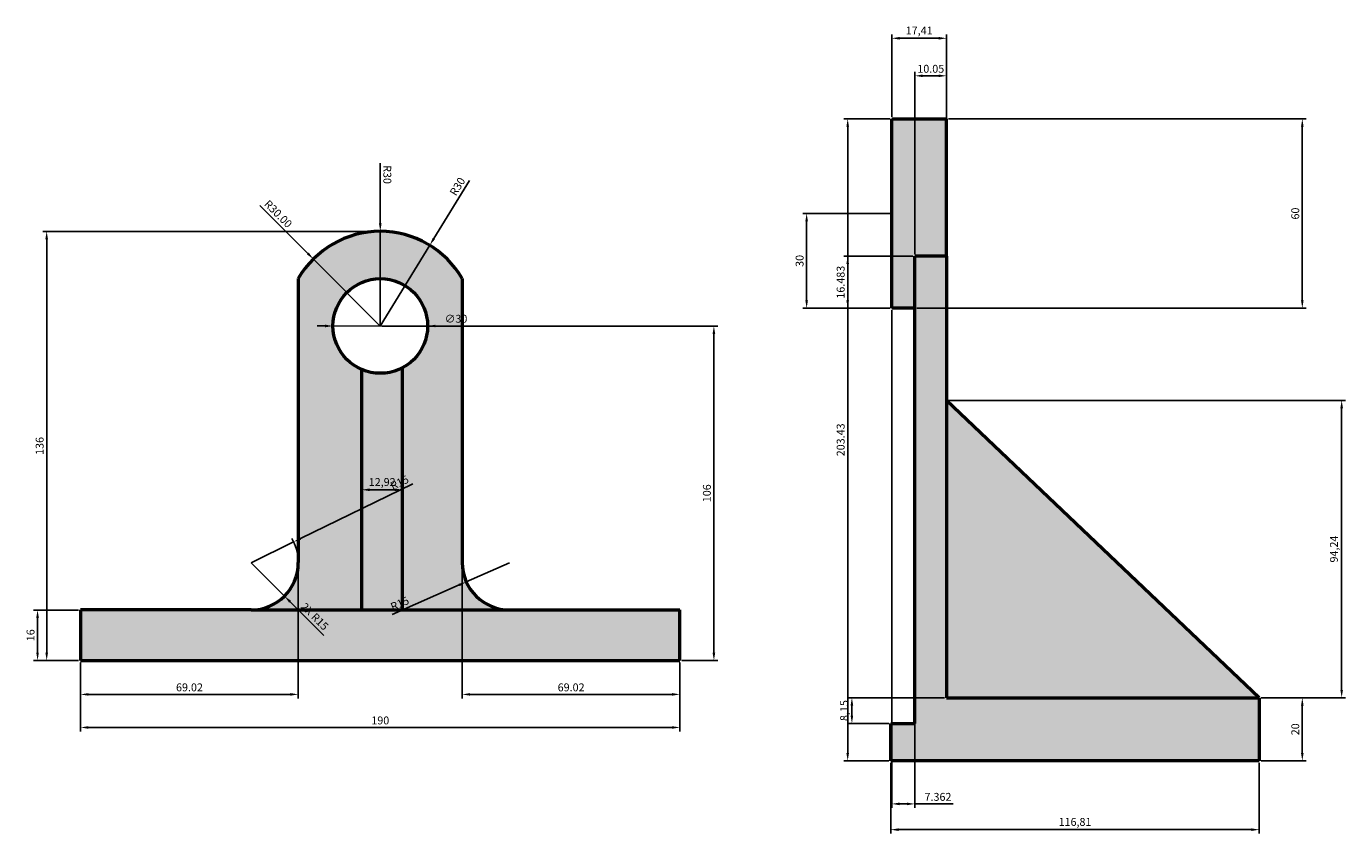
# Model space of a CAD drawing. Units: millimetres. Extents: x 1248 to 2192, y 1962 to 2325.
# Tile 4 of 4: x 1773 to 2192, y 2069 to 2325. Entities that reach past the tile are written whole.
import ezdxf

# ---------------------------------------------------------------- set-up
doc = ezdxf.new("R2010")
doc.units = ezdxf.units.MM
for name, color, linetype, lineweight in [('M-DIMS', 2, 'Continuous', 25), ('M-HATC', 8, 'Continuous', 18), ('M-OUTL', 7, 'Continuous', 50)]:
    doc.layers.add(name, color=color, linetype=linetype, lineweight=lineweight)
doc.styles.get("Standard").update_dxf_attribs({"font": 'arial.ttf'})
doc.dimstyles.new('ISO-25', dxfattribs={"dimtxt": 2.5, "dimasz": 2.5, "dimexe": 1.25, "dimexo": 0.625, "dimtad": 1, "dimtxsty": 'Standard', "dimcen": 2.5, "dimadec": 0, "dimazin": 0, "dimtfac": 1, "dimtmove": 0, "dimatfit": 3, "dimfxl": 1, "dimarcsym": 0})

# ---------------------------------------------------------------- blocks, each defined once
blk = doc.blocks.new('*D23')
at = {"layer": 'Defpoints', "color": 0, "transparency": 16777216}
for p in [(1790.51, 2124.07), (1980.51, 2124.07), (1980.51, 2102.85)]:
    blk.add_point(p, dxfattribs=at)
at = {"layer": 'M-DIMS', "color": 0, "lineweight": -2, "transparency": 16777216}
for p, q in [((1790.51, 2123.45), (1790.51, 2101.6)), ((1980.51, 2123.45), (1980.51, 2101.6)), ((1793.01, 2102.85), (1978.01, 2102.85))]:
    blk.add_line(p, q, dxfattribs=at)
at = {"layer": 'M-DIMS', "color": 0, "transparency": 16777216}
for points in [[(1793.01, 2103.26), (1793.01, 2102.43), (1790.51, 2102.85)], [(1978.01, 2103.26), (1978.01, 2102.43), (1980.51, 2102.85)]]:
    blk.add_solid(points, dxfattribs=at)
at = {"layer": 'M-DIMS', "color": 0, "transparency": 16777216, "insert": (1885.51, 2104.75), "char_height": 2.5, "attachment_point": 5}
blk.add_mtext('190', dxfattribs=at)
blk = doc.blocks.new('*D24')
at = {"layer": 'Defpoints', "color": 0, "transparency": 16777216}
for p in [(1776.87, 2140.07), (1790.51, 2140.07), (1790.51, 2124.07)]:
    blk.add_point(p, dxfattribs=at)
at = {"layer": 'M-DIMS', "color": 0, "lineweight": -2, "transparency": 16777216}
for p, q in [((1789.89, 2140.07), (1775.62, 2140.07)), ((1776.87, 2126.57), (1776.87, 2137.57)), ((1789.89, 2124.07), (1775.62, 2124.07))]:
    blk.add_line(p, q, dxfattribs=at)
at = {"layer": 'M-DIMS', "color": 0, "transparency": 16777216}
for points in [[(1776.45, 2137.57), (1777.28, 2137.57), (1776.87, 2140.07)], [(1776.45, 2126.57), (1777.28, 2126.57), (1776.87, 2124.07)]]:
    blk.add_solid(points, dxfattribs=at)
at = {"layer": 'M-DIMS', "color": 0, "transparency": 16777216, "insert": (1774.97, 2132.07), "char_height": 2.5, "attachment_point": 5, "rotation": 90}
blk.add_mtext('16', dxfattribs=at)
blk = doc.blocks.new('*D25')
at = {"layer": 'Defpoints', "color": 0, "transparency": 16777216}
for p in [(1901.18, 2255.66), (1885.51, 2230.07)]:
    blk.add_point(p, dxfattribs=at)
at = {"layer": 'M-DIMS', "color": 0, "lineweight": -2, "transparency": 16777216}
for p, q in [((1913.76, 2276.19), (1902.49, 2257.79)), ((1885.51, 2230.07), (1901.18, 2255.66))]:
    blk.add_line(p, q, dxfattribs=at)
at = {"layer": 'M-DIMS', "color": 0, "transparency": 16777216}
blk.add_solid([(1902.13, 2258.01), (1902.84, 2257.57), (1901.18, 2255.66)], dxfattribs=at)
at = {"layer": 'M-DIMS', "color": 0, "transparency": 16777216, "insert": (1910.25, 2274.11), "char_height": 2.5, "attachment_point": 5, "rotation": 58.5121}
blk.add_mtext('R30', dxfattribs=at)
blk = doc.blocks.new('*D26')
at = {"layer": 'Defpoints', "color": 0, "transparency": 16777216}
for p in [(1858.02, 2161.64), (1844.53, 2155.07)]:
    blk.add_point(p, dxfattribs=at)
at = {"layer": 'M-DIMS', "color": 0, "lineweight": -2, "transparency": 16777216}
for p, q in [((1895.83, 2180.04), (1860.26, 2162.73)), ((1844.53, 2155.07), (1858.02, 2161.64))]:
    blk.add_line(p, q, dxfattribs=at)
blk.add_arc((1844.53, 2155.07), 15, 2.3873, 30.7269, dxfattribs=at)
at = {"layer": 'M-DIMS', "color": 0, "transparency": 16777216}
blk.add_solid([(1860.08, 2163.11), (1860.45, 2162.36), (1858.02, 2161.64)], dxfattribs=at)
at = {"layer": 'M-DIMS', "color": 0, "transparency": 16777216, "insert": (1891.74, 2180.17), "char_height": 2.5, "attachment_point": 5, "rotation": 25.9523}
blk.add_mtext('R15', dxfattribs=at)
blk = doc.blocks.new('*D27')
at = {"layer": 'Defpoints', "color": 0, "transparency": 16777216}
for p in [(1926.49, 2155.07), (1912.77, 2149.01)]:
    blk.add_point(p, dxfattribs=at)
at = {"layer": 'M-DIMS', "color": 0, "lineweight": -2, "transparency": 16777216}
for p, q in [((1926.49, 2155.07), (1912.77, 2149.01)), ((1889.26, 2138.61), (1910.49, 2148))]:
    blk.add_line(p, q, dxfattribs=at)
at = {"layer": 'M-DIMS', "color": 0, "transparency": 16777216}
blk.add_solid([(1910.32, 2148.38), (1910.65, 2147.61), (1912.77, 2149.01)], dxfattribs=at)
at = {"layer": 'M-DIMS', "color": 0, "transparency": 16777216, "insert": (1891.81, 2141.81), "char_height": 2.5, "attachment_point": 5, "rotation": 23.8585}
blk.add_mtext('R15', dxfattribs=at)
blk = doc.blocks.new('*D28')
at = {"layer": 'Defpoints', "color": 0, "transparency": 16777216}
for p in [(1879.65, 2178.17), (1892.58, 2178.46), (1892.58, 2178.17)]:
    blk.add_point(p, dxfattribs=at)
at = {"layer": 'M-DIMS', "color": 0, "lineweight": -2, "transparency": 16777216}
for p, q in [((1879.65, 2178.8), (1879.65, 2179.42)), ((1882.15, 2178.17), (1890.08, 2178.17)), ((1892.58, 2177.83), (1892.58, 2176.92))]:
    blk.add_line(p, q, dxfattribs=at)
at = {"layer": 'M-DIMS', "color": 0, "transparency": 16777216}
for points in [[(1882.15, 2178.59), (1882.15, 2177.75), (1879.65, 2178.17)], [(1890.08, 2178.59), (1890.08, 2177.75), (1892.58, 2178.17)]]:
    blk.add_solid(points, dxfattribs=at)
at = {"layer": 'M-DIMS', "color": 0, "transparency": 16777216, "insert": (1886.11, 2180.3), "char_height": 2.5, "attachment_point": 5}
blk.add_mtext('12,92', dxfattribs=at)
blk = doc.blocks.new('*D29')
at = {"layer": 'Defpoints', "color": 0, "transparency": 16777216}
for p in [(2065.03, 2321.25), (2047.62, 2295.71), (2065.03, 2295.71)]:
    blk.add_point(p, dxfattribs=at)
at = {"layer": 'M-DIMS', "color": 0, "lineweight": -2, "transparency": 16777216}
for p, q in [((2047.62, 2296.33), (2047.62, 2322.5)), ((2050.12, 2321.25), (2062.53, 2321.25)), ((2065.03, 2296.33), (2065.03, 2322.5))]:
    blk.add_line(p, q, dxfattribs=at)
at = {"layer": 'M-DIMS', "color": 0, "transparency": 16777216}
for points in [[(2050.12, 2321.67), (2050.12, 2320.83), (2047.62, 2321.25)], [(2062.53, 2321.67), (2062.53, 2320.83), (2065.03, 2321.25)]]:
    blk.add_solid(points, dxfattribs=at)
at = {"layer": 'M-DIMS', "color": 0, "transparency": 16777216, "insert": (2056.32, 2323.38), "char_height": 2.5, "attachment_point": 5}
blk.add_mtext('17,41', dxfattribs=at)
blk = doc.blocks.new('*D30')
at = {"layer": 'Defpoints', "color": 0, "transparency": 16777216}
for p in [(2047.62, 2265.71), (2020.66, 2235.71), (2047.62, 2235.71)]:
    blk.add_point(p, dxfattribs=at)
at = {"layer": 'M-DIMS', "color": 0, "lineweight": -2, "transparency": 16777216}
for p, q in [((2046.99, 2265.71), (2019.41, 2265.71)), ((2020.66, 2263.21), (2020.66, 2238.21)), ((2046.99, 2235.71), (2019.41, 2235.71))]:
    blk.add_line(p, q, dxfattribs=at)
at = {"layer": 'M-DIMS', "color": 0, "transparency": 16777216}
for points in [[(2020.25, 2263.21), (2021.08, 2263.21), (2020.66, 2265.71)], [(2020.25, 2238.21), (2021.08, 2238.21), (2020.66, 2235.71)]]:
    blk.add_solid(points, dxfattribs=at)
at = {"layer": 'M-DIMS', "color": 0, "transparency": 16777216, "insert": (2018.76, 2250.71), "char_height": 2.5, "attachment_point": 5, "rotation": 90}
blk.add_mtext('30', dxfattribs=at)
blk = doc.blocks.new('*D31')
at = {"layer": 'Defpoints', "color": 0, "transparency": 16777216}
for p in [(2065.03, 2206.51), (2164.13, 2112.27), (2190.26, 2112.27)]:
    blk.add_point(p, dxfattribs=at)
at = {"layer": 'M-DIMS', "color": 0, "lineweight": -2, "transparency": 16777216}
for p, q in [((2065.66, 2206.51), (2191.51, 2206.51)), ((2190.26, 2204.01), (2190.26, 2114.77)), ((2164.76, 2112.27), (2191.51, 2112.27))]:
    blk.add_line(p, q, dxfattribs=at)
at = {"layer": 'M-DIMS', "color": 0, "transparency": 16777216}
for points in [[(2189.85, 2204.01), (2190.68, 2204.01), (2190.26, 2206.51)], [(2189.85, 2114.77), (2190.68, 2114.77), (2190.26, 2112.27)]]:
    blk.add_solid(points, dxfattribs=at)
at = {"layer": 'M-DIMS', "color": 0, "transparency": 16777216, "insert": (2188.13, 2159.39), "char_height": 2.5, "attachment_point": 5, "rotation": 90}
blk.add_mtext('94,24', dxfattribs=at)
blk = doc.blocks.new('*D32')
at = {"layer": 'Defpoints', "color": 0, "transparency": 16777216}
for p in [(2047.32, 2092.27), (2164.13, 2092.27), (2164.13, 2070.46)]:
    blk.add_point(p, dxfattribs=at)
at = {"layer": 'M-DIMS', "color": 0, "lineweight": -2, "transparency": 16777216}
for p, q in [((2047.32, 2091.65), (2047.32, 2069.21)), ((2164.13, 2091.65), (2164.13, 2069.21)), ((2049.82, 2070.46), (2161.63, 2070.46))]:
    blk.add_line(p, q, dxfattribs=at)
at = {"layer": 'M-DIMS', "color": 0, "transparency": 16777216}
for points in [[(2049.82, 2070.88), (2049.82, 2070.04), (2047.32, 2070.46)], [(2161.63, 2070.88), (2161.63, 2070.04), (2164.13, 2070.46)]]:
    blk.add_solid(points, dxfattribs=at)
at = {"layer": 'M-DIMS', "color": 0, "transparency": 16777216, "insert": (2105.73, 2072.59), "char_height": 2.5, "attachment_point": 5}
blk.add_mtext('116,81', dxfattribs=at)
blk = doc.blocks.new('*D33')
at = {"layer": 'Defpoints', "color": 0, "transparency": 16777216}
for p in [(2035.01, 2112.27), (2065.03, 2112.27), (2047.32, 2104.13)]:
    blk.add_point(p, dxfattribs=at)
at = {"layer": 'M-DIMS', "color": 0, "lineweight": -2, "transparency": 16777216}
for p, q in [((2064.41, 2112.27), (2033.76, 2112.27)), ((2035.01, 2106.63), (2035.01, 2109.77)), ((2046.7, 2104.13), (2033.76, 2104.13))]:
    blk.add_line(p, q, dxfattribs=at)
at = {"layer": 'M-DIMS', "color": 0, "transparency": 16777216}
for points in [[(2034.59, 2109.77), (2035.42, 2109.77), (2035.01, 2112.27)], [(2034.59, 2106.63), (2035.42, 2106.63), (2035.01, 2104.13)]]:
    blk.add_solid(points, dxfattribs=at)
at = {"layer": 'M-DIMS', "color": 0, "transparency": 16777216, "insert": (2032.88, 2108.2), "char_height": 2.5, "attachment_point": 5, "rotation": 90}
blk.add_mtext('8,15', dxfattribs=at)
blk = doc.blocks.new('*D34')
at = {"layer": 'Defpoints', "color": 0, "transparency": 16777216}
for p in [(1779.76, 2260.07), (1885.51, 2260.07), (1790.51, 2124.07)]:
    blk.add_point(p, dxfattribs=at)
at = {"layer": 'M-DIMS', "color": 0, "lineweight": -2, "transparency": 16777216}
for p, q in [((1884.89, 2260.07), (1778.51, 2260.07)), ((1779.76, 2126.57), (1779.76, 2257.57)), ((1789.89, 2124.07), (1778.51, 2124.07))]:
    blk.add_line(p, q, dxfattribs=at)
at = {"layer": 'M-DIMS', "color": 0, "transparency": 16777216}
for points in [[(1779.34, 2257.57), (1780.18, 2257.57), (1779.76, 2260.07)], [(1779.34, 2126.57), (1780.18, 2126.57), (1779.76, 2124.07)]]:
    blk.add_solid(points, dxfattribs=at)
at = {"layer": 'M-DIMS', "color": 0, "transparency": 16777216, "insert": (1777.86, 2192.07), "char_height": 2.5, "attachment_point": 5, "rotation": 90}
blk.add_mtext('136', dxfattribs=at)
blk = doc.blocks.new('*D35')
at = {"layer": 'Defpoints', "color": 0, "transparency": 16777216}
for p in [(1885.51, 2230.07), (1991.26, 2230.07), (1980.51, 2124.07)]:
    blk.add_point(p, dxfattribs=at)
at = {"layer": 'M-DIMS', "color": 0, "lineweight": -2, "transparency": 16777216}
for p, q in [((1886.14, 2230.07), (1992.51, 2230.07)), ((1991.26, 2126.57), (1991.26, 2227.57)), ((1981.14, 2124.07), (1992.51, 2124.07))]:
    blk.add_line(p, q, dxfattribs=at)
at = {"layer": 'M-DIMS', "color": 0, "transparency": 16777216}
for points in [[(1990.84, 2227.57), (1991.68, 2227.57), (1991.26, 2230.07)], [(1990.84, 2126.57), (1991.68, 2126.57), (1991.26, 2124.07)]]:
    blk.add_solid(points, dxfattribs=at)
at = {"layer": 'M-DIMS', "color": 0, "transparency": 16777216, "insert": (1989.36, 2177.07), "char_height": 2.5, "attachment_point": 5, "rotation": 90}
blk.add_mtext('106', dxfattribs=at)
blk = doc.blocks.new('*D36')
at = {"layer": 'Defpoints', "color": 0, "transparency": 16777216}
for p in [(1911.49, 2155.07), (1980.51, 2124.07), (1980.51, 2113.32)]:
    blk.add_point(p, dxfattribs=at)
at = {"layer": 'M-DIMS', "color": 0, "lineweight": -2, "transparency": 16777216}
for p, q in [((1911.49, 2154.45), (1911.49, 2112.07)), ((1980.51, 2123.45), (1980.51, 2112.07)), ((1913.99, 2113.32), (1978.01, 2113.32))]:
    blk.add_line(p, q, dxfattribs=at)
at = {"layer": 'M-DIMS', "color": 0, "transparency": 16777216}
for points in [[(1913.99, 2113.74), (1913.99, 2112.91), (1911.49, 2113.32)], [(1978.01, 2113.74), (1978.01, 2112.91), (1980.51, 2113.32)]]:
    blk.add_solid(points, dxfattribs=at)
at = {"layer": 'M-DIMS', "color": 0, "transparency": 16777216, "insert": (1946, 2115.23), "char_height": 2.5, "attachment_point": 5}
blk.add_mtext('69.02', dxfattribs=at)
blk = doc.blocks.new('*D37')
at = {"layer": 'Defpoints', "color": 0, "transparency": 16777216}
for p in [(1859.53, 2155.07), (1790.51, 2124.07), (1859.53, 2113.32)]:
    blk.add_point(p, dxfattribs=at)
at = {"layer": 'M-DIMS', "color": 0, "lineweight": -2, "transparency": 16777216}
for p, q in [((1859.53, 2154.45), (1859.53, 2112.07)), ((1790.51, 2123.45), (1790.51, 2112.07)), ((1793.01, 2113.32), (1857.03, 2113.32))]:
    blk.add_line(p, q, dxfattribs=at)
at = {"layer": 'M-DIMS', "color": 0, "transparency": 16777216}
for points in [[(1793.01, 2113.74), (1793.01, 2112.91), (1790.51, 2113.32)], [(1857.03, 2113.74), (1857.03, 2112.91), (1859.53, 2113.32)]]:
    blk.add_solid(points, dxfattribs=at)
at = {"layer": 'M-DIMS', "color": 0, "transparency": 16777216, "insert": (1825.02, 2115.23), "char_height": 2.5, "attachment_point": 5}
blk.add_mtext('69.02', dxfattribs=at)
blk = doc.blocks.new('*D50')
at = {"layer": 'Defpoints', "color": 0, "transparency": 16777216}
for p in [(2033.67, 2295.71), (2047.62, 2295.71), (2047.32, 2092.27)]:
    blk.add_point(p, dxfattribs=at)
at = {"layer": 'M-DIMS', "color": 0, "lineweight": -2, "transparency": 16777216}
for p, q in [((2046.99, 2295.71), (2032.42, 2295.71)), ((2033.67, 2094.77), (2033.67, 2293.21)), ((2046.7, 2092.27), (2032.42, 2092.27))]:
    blk.add_line(p, q, dxfattribs=at)
at = {"layer": 'M-DIMS', "color": 0, "transparency": 16777216}
for points in [[(2033.25, 2293.21), (2034.09, 2293.21), (2033.67, 2295.71)], [(2033.25, 2094.77), (2034.09, 2094.77), (2033.67, 2092.27)]]:
    blk.add_solid(points, dxfattribs=at)
at = {"layer": 'M-DIMS', "color": 0, "transparency": 16777216, "insert": (2031.77, 2193.99), "char_height": 2.5, "attachment_point": 5, "rotation": 90}
blk.add_mtext('203.43', dxfattribs=at)
blk = doc.blocks.new('*D51')
at = {"layer": 'Defpoints', "color": 0, "transparency": 16777216}
for p in [(2065.03, 2295.71), (2054.98, 2235.71), (2177.78, 2235.71)]:
    blk.add_point(p, dxfattribs=at)
at = {"layer": 'M-DIMS', "color": 0, "lineweight": -2, "transparency": 16777216}
for p, q in [((2065.66, 2295.71), (2179.03, 2295.71)), ((2177.78, 2293.21), (2177.78, 2238.21)), ((2055.61, 2235.71), (2179.03, 2235.71))]:
    blk.add_line(p, q, dxfattribs=at)
at = {"layer": 'M-DIMS', "color": 0, "transparency": 16777216}
for points in [[(2177.37, 2293.21), (2178.2, 2293.21), (2177.78, 2295.71)], [(2177.37, 2238.21), (2178.2, 2238.21), (2177.78, 2235.71)]]:
    blk.add_solid(points, dxfattribs=at)
at = {"layer": 'M-DIMS', "color": 0, "transparency": 16777216, "insert": (2175.88, 2265.71), "char_height": 2.5, "attachment_point": 5, "rotation": 90}
blk.add_mtext('60', dxfattribs=at)
blk = doc.blocks.new('*D52')
at = {"layer": 'Defpoints', "color": 0, "transparency": 16777216}
for p in [(2065.03, 2309.36), (2054.98, 2252.19), (2065.03, 2252.19)]:
    blk.add_point(p, dxfattribs=at)
at = {"layer": 'M-DIMS', "color": 0, "lineweight": -2, "transparency": 16777216}
for p, q in [((2054.98, 2252.81), (2054.98, 2310.61)), ((2057.48, 2309.36), (2062.53, 2309.36)), ((2065.03, 2252.81), (2065.03, 2310.61))]:
    blk.add_line(p, q, dxfattribs=at)
at = {"layer": 'M-DIMS', "color": 0, "transparency": 16777216}
for points in [[(2057.48, 2309.77), (2057.48, 2308.94), (2054.98, 2309.36)], [(2062.53, 2309.77), (2062.53, 2308.94), (2065.03, 2309.36)]]:
    blk.add_solid(points, dxfattribs=at)
at = {"layer": 'M-DIMS', "color": 0, "transparency": 16777216, "insert": (2060.01, 2311.26), "char_height": 2.5, "attachment_point": 5}
blk.add_mtext('10.05', dxfattribs=at)
blk = doc.blocks.new('*D53')
at = {"layer": 'Defpoints', "color": 0, "transparency": 16777216}
for p in [(2047.62, 2235.71), (2054.98, 2235.71), (2054.98, 2078.62)]:
    blk.add_point(p, dxfattribs=at)
at = {"layer": 'M-DIMS', "color": 0, "lineweight": -2, "transparency": 16777216}
for p, q in [((2047.62, 2235.08), (2047.62, 2077.37)), ((2054.98, 2235.08), (2054.98, 2077.37)), ((2050.12, 2078.62), (2052.48, 2078.62)), ((2054.98, 2078.62), (2067.12, 2078.62))]:
    blk.add_line(p, q, dxfattribs=at)
at = {"layer": 'M-DIMS', "color": 0, "transparency": 16777216}
for points in [[(2050.12, 2079.04), (2050.12, 2078.21), (2047.62, 2078.62)], [(2052.48, 2079.04), (2052.48, 2078.21), (2054.98, 2078.62)]]:
    blk.add_solid(points, dxfattribs=at)
at = {"layer": 'M-DIMS', "color": 0, "transparency": 16777216, "insert": (2062.3, 2080.53), "char_height": 2.5, "attachment_point": 5}
blk.add_mtext('7.362', dxfattribs=at)
blk = doc.blocks.new('*D54')
at = {"layer": 'Defpoints', "color": 0, "transparency": 16777216}
for p in [(2164.13, 2112.27), (2177.78, 2112.27), (2164.13, 2092.27)]:
    blk.add_point(p, dxfattribs=at)
at = {"layer": 'M-DIMS', "color": 0, "lineweight": -2, "transparency": 16777216}
for p, q in [((2164.76, 2112.27), (2179.03, 2112.27)), ((2177.78, 2094.77), (2177.78, 2109.77)), ((2164.76, 2092.27), (2179.03, 2092.27))]:
    blk.add_line(p, q, dxfattribs=at)
at = {"layer": 'M-DIMS', "color": 0, "transparency": 16777216}
for points in [[(2177.37, 2109.77), (2178.2, 2109.77), (2177.78, 2112.27)], [(2177.37, 2094.77), (2178.2, 2094.77), (2177.78, 2092.27)]]:
    blk.add_solid(points, dxfattribs=at)
at = {"layer": 'M-DIMS', "color": 0, "transparency": 16777216, "insert": (2175.88, 2102.27), "char_height": 2.5, "attachment_point": 5, "rotation": 90}
blk.add_mtext('20', dxfattribs=at)
blk = doc.blocks.new('*D55')
at = {"layer": 'Defpoints', "color": 0, "transparency": 16777216}
for p in [(2054.98, 2252.19), (2033.67, 2235.71), (2047.62, 2235.71)]:
    blk.add_point(p, dxfattribs=at)
at = {"layer": 'M-DIMS', "color": 0, "lineweight": -2, "transparency": 16777216}
for p, q in [((2054.36, 2252.19), (2032.42, 2252.19)), ((2033.67, 2249.69), (2033.67, 2238.21)), ((2046.99, 2235.71), (2032.42, 2235.71))]:
    blk.add_line(p, q, dxfattribs=at)
at = {"layer": 'M-DIMS', "color": 0, "transparency": 16777216}
for points in [[(2033.25, 2249.69), (2034.09, 2249.69), (2033.67, 2252.19)], [(2033.25, 2238.21), (2034.09, 2238.21), (2033.67, 2235.71)]]:
    blk.add_solid(points, dxfattribs=at)
at = {"layer": 'M-DIMS', "color": 0, "transparency": 16777216, "insert": (2031.77, 2243.95), "char_height": 2.5, "attachment_point": 5, "rotation": 90}
blk.add_mtext('16.483', dxfattribs=at)
blk = doc.blocks.new('*D57')
at = {"layer": 'Defpoints', "color": 0, "transparency": 16777216}
for p in [(1885.51, 2260.07), (1885.51, 2230.07)]:
    blk.add_point(p, dxfattribs=at)
at = {"layer": 'M-DIMS', "color": 0, "lineweight": -2, "transparency": 16777216}
for p, q in [((1885.51, 2281.68), (1885.51, 2262.57)), ((1885.51, 2230.07), (1885.51, 2260.07))]:
    blk.add_line(p, q, dxfattribs=at)
at = {"layer": 'M-DIMS', "color": 0, "transparency": 16777216}
blk.add_solid([(1885.93, 2262.57), (1885.09, 2262.57), (1885.51, 2260.07)], dxfattribs=at)
at = {"layer": 'M-DIMS', "color": 0, "transparency": 16777216, "insert": (1887.41, 2278.07), "char_height": 2.5, "attachment_point": 5, "rotation": 270.0005}
blk.add_mtext('R30', dxfattribs=at)
blk = doc.blocks.new('*D58')
at = {"layer": 'Defpoints', "color": 0, "transparency": 16777216}
for p in [(1844.53, 2155.07), (1855.14, 2144.47)]:
    blk.add_point(p, dxfattribs=at)
at = {"layer": 'M-DIMS', "color": 0, "lineweight": -2, "transparency": 16777216}
for p, q in [((1844.53, 2155.07), (1855.14, 2144.47)), ((1867.62, 2131.98), (1856.9, 2142.7))]:
    blk.add_line(p, q, dxfattribs=at)
at = {"layer": 'M-DIMS', "color": 0, "transparency": 16777216}
blk.add_solid([(1857.2, 2142.99), (1856.61, 2142.41), (1855.14, 2144.47)], dxfattribs=at)
at = {"layer": 'M-DIMS', "color": 0, "transparency": 16777216, "insert": (1864.49, 2137.8), "char_height": 2.5, "attachment_point": 5, "rotation": 315.0004}
blk.add_mtext('2X R15', dxfattribs=at)
blk = doc.blocks.new('*D59')
at = {"layer": 'Defpoints', "color": 0, "transparency": 16777216}
for p in [(1870.51, 2230.08), (1900.51, 2230.07)]:
    blk.add_point(p, dxfattribs=at)
at = {"layer": 'M-DIMS', "color": 0, "lineweight": -2, "transparency": 16777216}
for p, q in [((1868.01, 2230.08), (1865.51, 2230.08)), ((1870.51, 2230.08), (1900.51, 2230.07)), ((1913.28, 2230.07), (1903.01, 2230.07))]:
    blk.add_line(p, q, dxfattribs=at)
at = {"layer": 'M-DIMS', "color": 0, "transparency": 16777216}
for points in [[(1868.01, 2230.5), (1868.01, 2229.66), (1870.51, 2230.08)], [(1903.01, 2230.49), (1903.01, 2229.65), (1900.51, 2230.07)]]:
    blk.add_solid(points, dxfattribs=at)
at = {"layer": 'M-DIMS', "color": 0, "transparency": 16777216, "insert": (1909.51, 2232.04), "char_height": 2.5, "attachment_point": 5, "rotation": 359.9833}
blk.add_mtext('∅30', dxfattribs=at)
blk = doc.blocks.new('*D76')
at = {"layer": 'Defpoints', "color": 0, "transparency": 16777216}
for p in [(1864.3, 2251.3), (1885.51, 2230.07)]:
    blk.add_point(p, dxfattribs=at)
at = {"layer": 'M-DIMS', "color": 0, "lineweight": -2, "transparency": 16777216}
for p, q in [((1847.32, 2268.3), (1862.54, 2253.06)), ((1885.51, 2230.07), (1864.3, 2251.3))]:
    blk.add_line(p, q, dxfattribs=at)
at = {"layer": 'M-DIMS', "color": 0, "transparency": 16777216}
blk.add_solid([(1862.83, 2253.36), (1862.24, 2252.77), (1864.3, 2251.3)], dxfattribs=at)
at = {"layer": 'M-DIMS', "color": 0, "transparency": 16777216, "insert": (1852.93, 2265.37), "char_height": 2.5, "attachment_point": 5, "rotation": 314.9792}
blk.add_mtext('R30.00', dxfattribs=at)

msp = doc.modelspace()

# ---------------------------------------------------------------- hatches: boundary and pattern name
at = {"layer": 'M-HATC'}
h = msp.add_hatch(color=256, dxfattribs=at)
h.set_gradient(color1=(19, 103, 52), color2=(19, 103, 52))
h.paths.add_polyline_path([(2065.0307, 2295.7054), (2047.6192, 2295.7054), (2047.6192, 2235.7054), (2054.9809, 2235.7054), (2054.9809, 2252.1885), (2065.0307, 2252.1885)])
h.paths.add_polyline_path([(2065.0307, 2252.1885), (2054.9809, 2252.1885), (2054.9809, 2235.7054), (2054.9809, 2104.1278), (2047.3208, 2104.1278), (2047.3208, 2092.2737), (2164.1341, 2092.2737), (2164.1341, 2112.2737), (2065.0307, 2112.2737)])
h.paths.add_polyline_path([(2065.0307, 2206.5089), (2065.0307, 2112.2737), (2164.1341, 2112.2737)], flags=17)
h = msp.add_hatch(color=256, dxfattribs=at)
h.set_gradient(color1=(19, 103, 52), color2=(19, 103, 52))
h.paths.add_polyline_path([(1900.5102, 2230.0744, -0.276856), (1892.5754, 2216.8424), (1892.5754, 2140.0744), (1926.491, 2140.0744, -0.41421356), (1911.491, 2155.0744), (1911.491, 2245.0744, 0.57735027), (1859.5295, 2245.0744), (1859.5295, 2155.0744, -0.41421356), (1844.5295, 2140.0744), (1879.6505, 2140.0744), (1879.6505, 2216.2663, -0.30098911), (1870.5102, 2230.0744, -1)])
h.paths.add_polyline_path([(1892.5754, 2216.8424, -0.22671193), (1879.6505, 2216.2663), (1879.6505, 2140.0744), (1892.5754, 2140.0744)], flags=17)
h.paths.add_polyline_path([(1980.5102, 2140.0744), (1926.491, 2140.0744), (1892.5754, 2140.0744), (1844.5295, 2140.0744), (1790.5102, 2140.0744), (1790.5102, 2124.0744), (1980.5102, 2124.0744)])
h.paths.add_polyline_path([(1889.3776, 2176.1264), (1896.2624, 2179.4772), (1894.0079, 2184.1095), (1887.1231, 2180.7586)], flags=25)
h.paths.add_polyline_path([(1889.2946, 2137.8607), (1896.2972, 2140.9578), (1894.2134, 2145.6693), (1887.2108, 2142.5723)], flags=9)
h.paths.add_polyline_path([(1881.02, 2177.9248), (1891.0097, 2177.9248), (1891.0097, 2183.0766), (1881.02, 2183.0766)], flags=24)

# ---------------------------------------------------------------- linework, layer by layer
at = {"layer": 'M-OUTL'}
for p, q in [((2047.6192, 2235.7054), (2047.6192, 2295.7054)), ((2047.6192, 2295.7054), (2065.0307, 2295.7054)), ((2065.0307, 2252.1885), (2065.0307, 2295.7054)), ((2054.9809, 2104.1278), (2054.9809, 2252.1885)), ((2065.0307, 2252.1885), (2054.9809, 2252.1885)), ((2065.0307, 2252.1885), (2065.0307, 2112.2737)), ((1859.5295, 2245.0744), (1859.5295, 2155.0744)), ((1911.491, 2245.0744), (1911.491, 2155.0744)), ((2054.9809, 2235.7054), (2047.6192, 2235.7054)), ((1892.5754, 2140.0744), (1892.5754, 2216.8424)), ((1879.6505, 2140.0744), (1879.6505, 2216.2663)), ((2164.1341, 2112.2737), (2065.0307, 2206.5089)), ((1844.5295, 2140.0744), (1790.5102, 2140.0744)), ((1790.5102, 2140.0744), (1790.5102, 2124.0744)), ((1844.5295, 2140.0744), (1926.491, 2140.0744)), ((1926.491, 2140.0744), (1980.5102, 2140.0744)), ((1980.5102, 2124.0744), (1980.5102, 2140.0744)), ((1790.5102, 2124.0744), (1980.5102, 2124.0744)), ((2065.0307, 2112.2737), (2164.1341, 2112.2737)), ((2164.1341, 2112.2737), (2164.1341, 2092.2737)), ((2047.3208, 2092.2737), (2047.3208, 2104.1278)), ((2047.3208, 2104.1278), (2054.9809, 2104.1278)), ((2164.1341, 2092.2737), (2047.3208, 2092.2737))]:
    msp.add_line(p, q, dxfattribs=at)
msp.add_circle((1885.5102, 2230.0744), 15, dxfattribs=at)
for centre, radius, start, end in [((1885.5102, 2230.0744), 30, 30, 150), ((1844.5295, 2155.0744), 15, 270, 0), ((1926.491, 2155.0744), 15, 180, 270)]:
    msp.add_arc(centre, radius, start, end, dxfattribs=at)

# ---------------------------------------------------------------- dimensions: what is measured, and where the dimension line sits
at = {"layer": 'M-DIMS'}
for base, p1, p2, override, picture, middle in [((2065.0307, 2321.2507), (2047.6192, 2295.7054), (2065.0307, 2295.7054), {"dimclrd": 0, "dimclre": 0, "dimclrt": 0}, '*D29', (2056.325, 2323.3781)), ((2065.0307, 2309.3554), (2054.9809, 2252.1885), (2065.0307, 2252.1885), {"dimdec": 2, "dimlfac": 1, "dimrnd": 0, "dimzin": 0, "dimdsep": 46, "dimlunit": 2}, '*D52', (2060.0058, 2311.2569)), ((2054.9809, 2078.6237), (2047.6192, 2235.7054), (2054.9809, 2235.7054), {"dimdec": 3, "dimlfac": 1, "dimrnd": 0, "dimzin": 0, "dimdsep": 46, "dimlunit": 2}, '*D53', (2062.301, 2080.526)), ((1892.5754, 2178.1703), (1879.6505, 2178.1703), (1892.5754, 2178.4584), {"dimclrd": 0, "dimclre": 0, "dimclrt": 0}, '*D28', (1886.1129, 2180.2977)), ((1859.5295, 2113.3244), (1790.5102, 2124.0744), (1859.5295, 2155.0744), {"dimdec": 2, "dimlfac": 1, "dimrnd": 0, "dimzin": 0, "dimdsep": 46, "dimlunit": 2}, '*D37', (1825.0199, 2115.2258)), ((1980.5102, 2113.3244), (1911.491, 2155.0744), (1980.5102, 2124.0744), {"dimdec": 2, "dimlfac": 1, "dimrnd": 0, "dimzin": 0, "dimdsep": 46, "dimlunit": 2}, '*D36', (1946.0006, 2115.2258)), ((1980.5102, 2102.8459), (1790.5102, 2124.0744), (1980.5102, 2124.0744), {"dimclrd": 0, "dimclre": 0, "dimclrt": 0}, '*D23', (1885.5102, 2104.7473)), ((2164.1341, 2070.4605), (2047.3208, 2092.2737), (2164.1341, 2092.2737), {"dimclrd": 0, "dimclre": 0, "dimclrt": 0}, '*D32', (2105.7274, 2072.5879))]:
    dim = msp.add_linear_dim(base=base, p1=p1, p2=p2, dimstyle='ISO-25', override=override, dxfattribs=at)
    dim.commit()
    dim.dimension.update_dxf_attribs({"geometry": picture, "text_midpoint": middle})
for base, p1, p2, override, picture, middle in [((2033.6708, 2295.7054), (2047.3208, 2092.2737), (2047.6192, 2295.7054), {"dimdec": 2, "dimlfac": 1, "dimrnd": 0, "dimzin": 0, "dimdsep": 46, "dimlunit": 2}, '*D50', (2031.7685, 2193.9896)), ((2177.7841, 2235.7054), (2065.0307, 2295.7054), (2054.9809, 2235.7054), {"dimdec": 0, "dimlfac": 1, "dimrnd": 0, "dimzin": 0, "dimdsep": 46, "dimlunit": 2}, '*D51', (2175.8826, 2265.7054)), ((2020.6645, 2235.7054), (2047.6192, 2265.7054), (2047.6192, 2235.7054), {"dimclrd": 0, "dimclre": 0, "dimclrt": 0}, '*D30', (2018.7622, 2250.7054)), ((1779.7602, 2260.0744), (1790.5102, 2124.0744), (1885.5102, 2260.0744), {"dimdec": 0, "dimlfac": 1, "dimrnd": 0, "dimzin": 0, "dimdsep": 46, "dimlunit": 2}, '*D34', (1777.858, 2192.0744)), ((2033.6708, 2235.7054), (2054.9809, 2252.1885), (2047.6192, 2235.7054), {"dimdec": 3, "dimlfac": 1, "dimrnd": 0, "dimzin": 0, "dimdsep": 46, "dimlunit": 2}, '*D55', (2031.7685, 2243.947)), ((1991.2602, 2230.0744), (1980.5102, 2124.0744), (1885.5102, 2230.0744), {"dimdec": 0, "dimlfac": 1, "dimrnd": 0, "dimzin": 0, "dimdsep": 46, "dimlunit": 2}, '*D35', (1989.3588, 2177.0744)), ((2190.2619, 2112.2737), (2065.0307, 2206.5089), (2164.1341, 2112.2737), {"dimclrd": 0, "dimclre": 0, "dimclrt": 0}, '*D31', (2188.1345, 2159.3913)), ((1776.8667, 2140.0744), (1790.5102, 2124.0744), (1790.5102, 2140.0744), {"dimclrd": 0, "dimclre": 0, "dimclrt": 0}, '*D24', (1774.9653, 2132.0744)), ((2035.0073, 2112.2737), (2047.3208, 2104.1278), (2065.0307, 2112.2737), {"dimclrd": 0, "dimclre": 0, "dimclrt": 0}, '*D33', (2032.8799, 2108.2008)), ((2177.7841, 2112.2737), (2164.1341, 2092.2737), (2164.1341, 2112.2737), {"dimdec": 0, "dimlfac": 1, "dimrnd": 0, "dimzin": 0, "dimdsep": 46, "dimlunit": 2}, '*D54', (2175.8826, 2102.2737))]:
    dim = msp.add_linear_dim(base=base, p1=p1, p2=p2, angle=90, dimstyle='ISO-25', override=override, dxfattribs=at)
    dim.commit()
    dim.dimension.update_dxf_attribs({"geometry": picture, "text_midpoint": middle})
for center, mpoint, override, picture, middle in [((1885.5102, 2230.0744), (1885.51, 2260.0744), {"dimdec": 0, "dimlfac": 1, "dimrnd": 0, "dimzin": 0, "dimdsep": 46, "dimlunit": 2}, '*D57', (1885.5099, 2278.0744)), ((1885.5102, 2230.0744), (1901.1798, 2255.6569), {"dimclrd": 0, "dimclre": 0, "dimclrt": 0}, '*D25', (1911.8719, 2273.1131)), ((1885.5102, 2230.0744), (1864.3047, 2251.2953), {"dimdec": 2, "dimlfac": 1, "dimrnd": 0, "dimzin": 0, "dimdsep": 46, "dimlunit": 2}, '*D76', (1851.5814, 2264.0278)), ((1844.5295, 2155.0744), (1858.0169, 2161.6387), {"dimclrd": 0, "dimclre": 0, "dimclrt": 0}, '*D26', (1892.5754, 2178.4584)), ((1926.491, 2155.0744), (1912.7728, 2149.0072), {"dimclrd": 0, "dimclre": 0, "dimclrt": 0}, '*D27', (1892.5754, 2140.0744))]:
    dim = msp.add_radius_dim(center=center, mpoint=mpoint, dimstyle='ISO-25', override=override, dxfattribs=at)
    dim.commit()
    dim.dimension.update_dxf_attribs({"geometry": picture, "text_midpoint": middle, "dimtype": 164})
dim = msp.add_diameter_dim_2p(p1=(1870.5102, 2230.0788), p2=(1900.5102, 2230.07), dimstyle='ISO-25', override={"dimdec": 0, "dimlfac": 1, "dimrnd": 0, "dimzin": 0, "dimdsep": 46, "dimlunit": 2}, dxfattribs=at)
dim.commit()
dim.dimension.update_dxf_attribs({"geometry": '*D59', "text_midpoint": (1909.5102, 2230.0674), "dimtype": 163})
dim = msp.add_radius_dim(center=(1844.5295, 2155.0744), mpoint=(1855.1361, 2144.4679), text='2X <>', dimstyle='ISO-25', override={"dimdec": 0, "dimlfac": 1, "dimrnd": 0, "dimzin": 0, "dimdsep": 46, "dimlunit": 2}, dxfattribs=at)
dim.commit()
dim.dimension.update_dxf_attribs({"geometry": '*D58', "text_midpoint": (1864.4911, 2137.802)})

doc.saveas('drawing.dxf')
